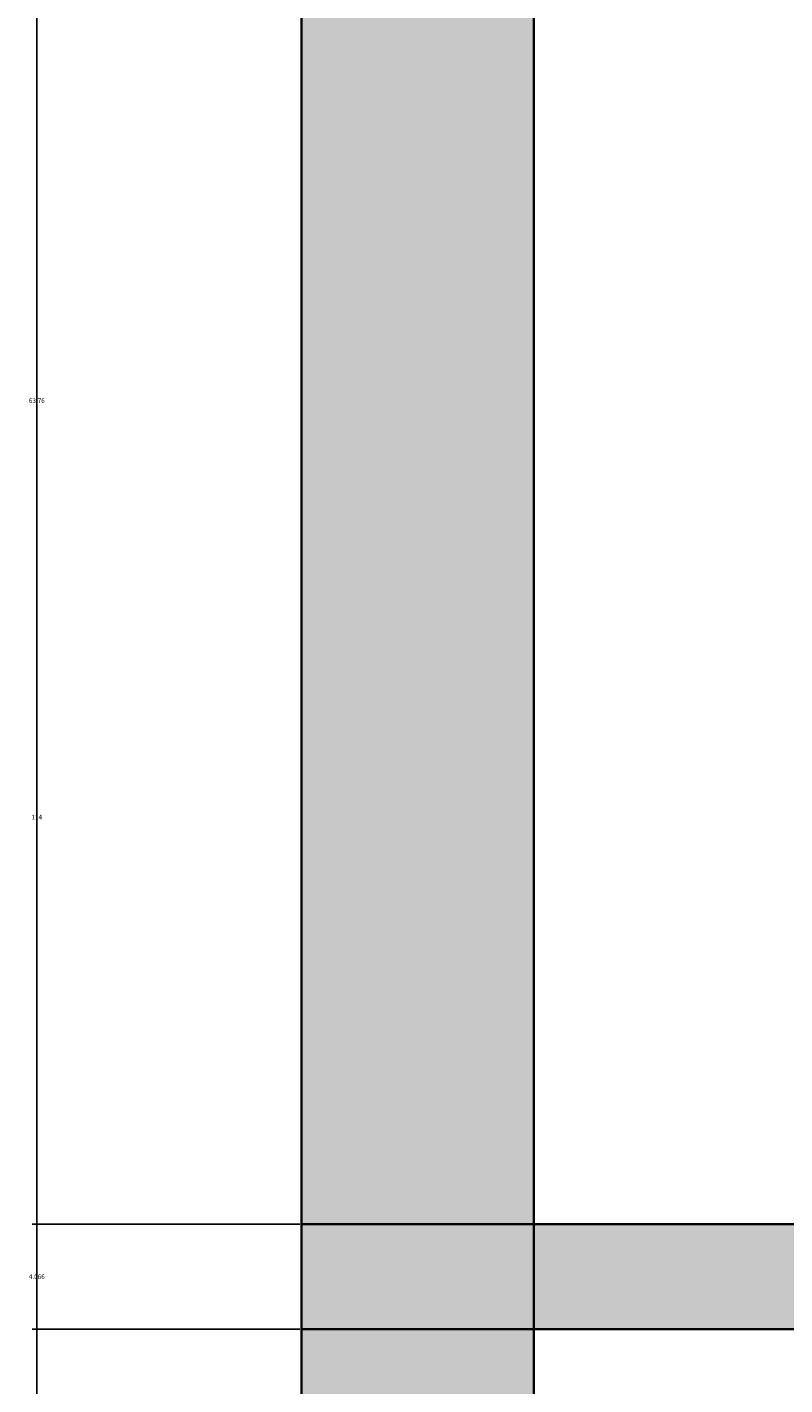
# Model space of a CAD drawing. Units: millimetres. Extents: x 446512 to 447461, y 70395 to 70610.
# Tile 23 of 39: x 446954 to 446983, y 70477 to 70530. Entities that reach past the tile are written whole.
import ezdxf

# ---------------------------------------------------------------- set-up
doc = ezdxf.new("R2010")
doc.units = ezdxf.units.MM
for name, color, linetype, lineweight in [('A-ANNO-DIMS', 2, 'Continuous', 18), ('A-FURN', 7, 'Continuous', 35), ('A-FURN-PATT', 38, 'Continuous', 13)]:
    doc.layers.add(name, color=color, linetype=linetype, lineweight=lineweight)
doc.styles.get("Standard").update_dxf_attribs({"font": 'arial.ttf'})
doc.dimstyles.get("Standard").update_dxf_attribs({"dimtxt": 0.18, "dimasz": 0.18, "dimexe": 0.18, "dimexo": 0.0625, "dimgap": 0.09, "dimtad": 0, "dimtih": 1, "dimtoh": 1, "dimdec": 4, "dimzin": 0, "dimdsep": 46, "dimtxsty": 'Standard', "dimcen": 0.09, "dimadec": 0, "dimazin": 0, "dimtfac": 1, "dimtdec": 4, "dimtofl": 0, "dimtmove": 0, "dimatfit": 3, "dimfxl": 1, "dimtolj": 1, "dimtzin": 0, "dimarcsym": 0})

# ---------------------------------------------------------------- blocks, each defined once
blk = doc.blocks.new('*D54')
at = {"layer": 'A-ANNO-DIMS', "color": 0, "lineweight": -2, "transparency": 16777216}
for p, q in [((446964.107, 70556.451), (446953.739, 70556.451)), ((446953.919, 70556.271), (446953.919, 70499.631)), ((446953.919, 70442.631), (446953.919, 70499.27)), ((446964.107, 70442.451), (446953.739, 70442.451))]:
    blk.add_line(p, q, dxfattribs=at)
at = {"layer": 'A-ANNO-DIMS', "color": 0, "transparency": 16777216}
for points in [[(446953.889, 70556.271), (446953.949, 70556.271), (446953.919, 70556.451)], [(446953.889, 70442.631), (446953.949, 70442.631), (446953.919, 70442.451)]]:
    blk.add_solid(points, dxfattribs=at)
at = {"layer": 'Defpoints', "color": 0, "transparency": 16777216}
for p in [(446953.919, 70556.451), (446964.169, 70556.451), (446964.169, 70442.451)]:
    blk.add_point(p, dxfattribs=at)
at = {"layer": 'A-ANNO-DIMS', "color": 0, "transparency": 16777216, "insert": (446953.919, 70499.451), "char_height": 0.18, "attachment_point": 5}
blk.add_mtext('\\A1;114', dxfattribs=at)
blk = doc.blocks.new('*D57')
at = {"layer": 'A-ANNO-DIMS', "color": 0, "lineweight": -2, "transparency": 16777216}
for p, q in [((446964.107, 70479.627), (446953.739, 70479.627)), ((446953.919, 70479.447), (446953.919, 70465.721)), ((446953.919, 70451.631), (446953.919, 70465.357)), ((446973.107, 70451.451), (446953.739, 70451.451))]:
    blk.add_line(p, q, dxfattribs=at)
at = {"layer": 'A-ANNO-DIMS', "color": 0, "transparency": 16777216}
for points in [[(446953.889, 70479.447), (446953.949, 70479.447), (446953.919, 70479.627)], [(446953.889, 70451.631), (446953.949, 70451.631), (446953.919, 70451.451)]]:
    blk.add_solid(points, dxfattribs=at)
at = {"layer": 'Defpoints', "color": 0, "transparency": 16777216}
for p in [(446953.919, 70479.627), (446964.169, 70479.627), (446973.169, 70451.451)]:
    blk.add_point(p, dxfattribs=at)
at = {"layer": 'A-ANNO-DIMS', "color": 0, "transparency": 16777216, "insert": (446953.919, 70465.539), "char_height": 0.18, "attachment_point": 5}
blk.add_mtext('\\A1;28.176', dxfattribs=at)
blk = doc.blocks.new('*D58')
at = {"layer": 'A-ANNO-DIMS', "color": 0, "lineweight": -2, "transparency": 16777216}
for p, q in [((446964.107, 70483.693), (446953.739, 70483.693)), ((446953.919, 70483.513), (446953.919, 70481.842)), ((446953.919, 70479.807), (446953.919, 70481.478)), ((446964.107, 70479.627), (446953.739, 70479.627))]:
    blk.add_line(p, q, dxfattribs=at)
at = {"layer": 'A-ANNO-DIMS', "color": 0, "transparency": 16777216}
for points in [[(446953.889, 70483.513), (446953.949, 70483.513), (446953.919, 70483.693)], [(446953.889, 70479.807), (446953.949, 70479.807), (446953.919, 70479.627)]]:
    blk.add_solid(points, dxfattribs=at)
at = {"layer": 'Defpoints', "color": 0, "transparency": 16777216}
for p in [(446953.919, 70483.693), (446964.169, 70483.693), (446964.169, 70479.627)]:
    blk.add_point(p, dxfattribs=at)
at = {"layer": 'A-ANNO-DIMS', "color": 0, "transparency": 16777216, "insert": (446953.919, 70481.66), "char_height": 0.18, "attachment_point": 5}
blk.add_mtext('\\A1;4.066', dxfattribs=at)
blk = doc.blocks.new('*D59')
at = {"layer": 'A-ANNO-DIMS', "color": 0, "lineweight": -2, "transparency": 16777216}
for p, q in [((446973.107, 70547.451), (446953.739, 70547.451)), ((446953.919, 70547.271), (446953.919, 70515.754)), ((446953.919, 70483.873), (446953.919, 70515.39)), ((446964.107, 70483.693), (446953.739, 70483.693))]:
    blk.add_line(p, q, dxfattribs=at)
at = {"layer": 'A-ANNO-DIMS', "color": 0, "transparency": 16777216}
for points in [[(446953.889, 70547.271), (446953.949, 70547.271), (446953.919, 70547.451)], [(446953.889, 70483.873), (446953.949, 70483.873), (446953.919, 70483.693)]]:
    blk.add_solid(points, dxfattribs=at)
at = {"layer": 'Defpoints', "color": 0, "transparency": 16777216}
for p in [(446953.919, 70547.451), (446973.169, 70547.451), (446964.169, 70483.693)]:
    blk.add_point(p, dxfattribs=at)
at = {"layer": 'A-ANNO-DIMS', "color": 0, "transparency": 16777216, "insert": (446953.919, 70515.572), "char_height": 0.18, "attachment_point": 5}
blk.add_mtext('\\A1;63.76', dxfattribs=at)

msp = doc.modelspace()

# ---------------------------------------------------------------- hatches: boundary and pattern name
at = {"layer": 'A-FURN-PATT'}
h = msp.add_hatch(color=256, dxfattribs=at)
h.dxf.hatch_style = 1
h.paths.add_polyline_path([(446983.5069, 70556.4508), (446964.1693, 70556.4508), (446964.1693, 70442.4508), (446983.5069, 70442.4508), (446983.5069, 70451.4508), (446973.1693, 70451.4508), (446973.1693, 70547.4508), (446983.5069, 70547.4508)])
h.paths.add_polyline_path([(447030.1693, 70556.4508), (446983.5069, 70556.4508), (446983.5069, 70547.4508), (447021.1693, 70547.4508), (447021.1693, 70451.4508), (446983.5069, 70451.4508), (446983.5069, 70442.4508), (447030.1693, 70442.4508)])
h = msp.add_hatch(color=256, dxfattribs=at)
h.dxf.hatch_style = 1
h.paths.add_polyline_path([(446973.1693, 70483.6935), (446964.1693, 70483.6935), (446964.1693, 70479.6272), (446973.1693, 70479.6272)])
h = msp.add_hatch(color=256, dxfattribs=at)
h.dxf.hatch_style = 1
h.paths.add_polyline_path([(446983.5069, 70483.6935), (446973.1693, 70483.6935), (446973.1693, 70479.6272), (446983.5069, 70479.6272)])

# ---------------------------------------------------------------- linework, layer by layer
at = {"layer": 'A-FURN'}
for points in [[(447030.1693, 70556.4508), (447030.1693, 70442.4508), (446964.1693, 70442.4508), (446964.1693, 70556.4508)], [(447021.1693, 70547.4508), (447021.1693, 70451.4508), (446973.1693, 70451.4508), (446973.1693, 70547.4508)], [(446964.1693, 70483.6935), (447030.1693, 70483.6935), (447030.1693, 70479.6272), (446964.1693, 70479.6272)]]:
    msp.add_lwpolyline(points, close=True, dxfattribs=at)

# ---------------------------------------------------------------- dimensions: what is measured, and where the dimension line sits
at = {"layer": 'A-ANNO-DIMS'}
for base, p1, p2, override, picture, middle in [((446953.9193, 70556.4508), (446964.1693, 70442.4508), (446964.1693, 70556.4508), {"dimdec": 0, "dimlfac": 1, "dimrnd": 0, "dimzin": 0, "dimdsep": 46, "dimlunit": 2}, '*D54', (446953.9193, 70499.4508)), ((446953.9193, 70547.4508), (446964.1693, 70483.6935), (446973.1693, 70547.4508), {"dimdec": 2, "dimlfac": 1, "dimrnd": 0, "dimzin": 0, "dimdsep": 46, "dimlunit": 2}, '*D59', (446953.9193, 70515.5721)), ((446953.9193, 70483.6935), (446964.1693, 70479.6272), (446964.1693, 70483.6935), {"dimdec": 3, "dimlfac": 1, "dimrnd": 0, "dimzin": 0, "dimdsep": 46, "dimlunit": 2}, '*D58', (446953.9193, 70481.6604)), ((446953.9193, 70479.6272), (446973.1693, 70451.4508), (446964.1693, 70479.6272), {"dimdec": 3, "dimlfac": 1, "dimrnd": 0, "dimzin": 0, "dimdsep": 46, "dimlunit": 2}, '*D57', (446953.9193, 70465.539))]:
    dim = msp.add_linear_dim(base=base, p1=p1, p2=p2, angle=90, dimstyle='Standard', override=override, dxfattribs=at)
    dim.commit()
    dim.dimension.update_dxf_attribs({"geometry": picture, "text_midpoint": middle})

doc.saveas('drawing.dxf')
